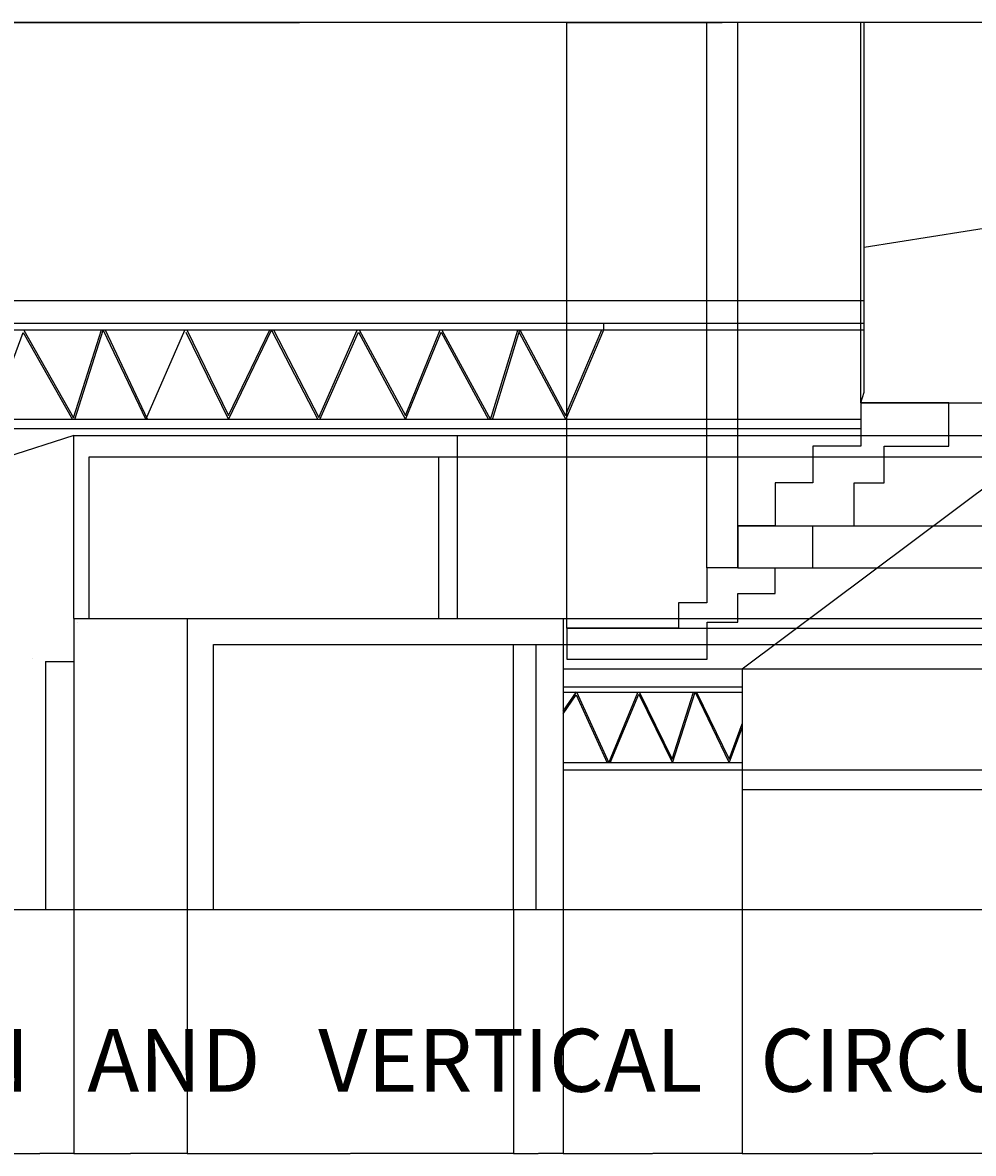
# Model space of a CAD drawing. Units: inches. Extents: x -32109 to 33221, y -19197 to 7608.
# Tile 24 of 25: x 19011 to 26633, y -13530 to -4467. Entities that reach past the tile are written whole.
import ezdxf

# ---------------------------------------------------------------- set-up
doc = ezdxf.new("R2010")
doc.units = ezdxf.units.IN
doc.header["$MEASUREMENT"] = 0
for name, color, linetype, lineweight in [('A-ANNO-DIMS', 2, 'Continuous', 18), ('A-ANNO-TEXT', 7, 'Continuous', 25), ('A-ELEV', 7, 'Continuous', 25)]:
    doc.layers.add(name, color=color, linetype=linetype, lineweight=lineweight)
doc.styles.get("Standard").update_dxf_attribs({"font": 'arial.ttf'})
doc.dimstyles.get("Standard").update_dxf_attribs({"dimtxt": 0.18, "dimasz": 0.18, "dimexe": 0.18, "dimexo": 0.0625, "dimgap": 0.09, "dimtad": 0, "dimtih": 1, "dimtoh": 1, "dimdec": 4, "dimzin": 0, "dimdsep": 46, "dimtxsty": 'Standard', "dimcen": 0.09, "dimadec": 0, "dimazin": 0, "dimtfac": 1, "dimtdec": 4, "dimtofl": 0, "dimtmove": 0, "dimatfit": 3, "dimfxl": 1, "dimtolj": 1, "dimtzin": 0, "dimarcsym": 0})

# ---------------------------------------------------------------- blocks, each defined once
blk = doc.blocks.new('*D16')
at = {"layer": 'A-ANNO-DIMS', "color": 0, "lineweight": -2, "transparency": 16777216}
for p, q in [((7931.85712, -8929.002357), (7931.85712, -4467.086268999999)), ((7932.03712, -4467.266268999999), (18774.66361096794, -4467.266268999999)), ((29618.150443, -4467.266268999999), (18775.52395203206, -4467.266268999999)), ((29618.330443, -6090.731526999999), (29618.330443, -4467.086268999999))]:
    blk.add_line(p, q, dxfattribs=at)
at = {"layer": 'A-ANNO-DIMS', "color": 0, "transparency": 16777216}
for points in [[(7932.03712, -4467.236268999999), (7932.03712, -4467.296269), (7931.85712, -4467.266268999999)], [(29618.150443, -4467.236268999999), (29618.150443, -4467.296269), (29618.330443, -4467.266268999999)]]:
    blk.add_solid(points, dxfattribs=at)
at = {"layer": 'Defpoints', "color": 0, "transparency": 16777216}
for p in [(29618.330443, -4467.266268999999), (29618.330443, -6090.794027), (7931.85712, -8929.064857)]:
    blk.add_point(p, dxfattribs=at)
at = {"layer": 'A-ANNO-DIMS', "color": 0, "transparency": 16777216, "insert": (18775.0937815, -4467.266268999999), "char_height": 0.18, "attachment_point": 5}
blk.add_mtext('\\A1;21686', dxfattribs=at)
blk = doc.blocks.new('*D17')
at = {"layer": 'A-ANNO-DIMS', "color": 0, "lineweight": -2, "transparency": 16777216}
for p, q in [((29618.39294300002, -6090.794027000002), (33221.11530000003, -6090.794027000001)), ((33220.93530000003, -6090.974027000001), (33220.93530000003, -8833.116883862214)), ((33220.93530000003, -11575.623547), (33220.93530000003, -8833.48069013779)), ((8978.174905000003, -11575.803547), (33221.11530000003, -11575.803547))]:
    blk.add_line(p, q, dxfattribs=at)
at = {"layer": 'A-ANNO-DIMS', "color": 0, "transparency": 16777216}
for points in [[(33220.90530000003, -6090.974027000001), (33220.96530000003, -6090.974027000001), (33220.93530000003, -6090.794027000001)], [(33220.90530000003, -11575.623547), (33220.96530000003, -11575.623547), (33220.93530000003, -11575.803547)]]:
    blk.add_solid(points, dxfattribs=at)
at = {"layer": 'Defpoints', "color": 0, "transparency": 16777216}
for p in [(29618.33044300001, -6090.794027000002), (8978.112405000002, -11575.803547), (33220.93530000003, -11575.803547)]:
    blk.add_point(p, dxfattribs=at)
at = {"layer": 'A-ANNO-DIMS', "color": 0, "transparency": 16777216, "insert": (33220.93530000002, -8833.298787000009), "char_height": 0.18, "attachment_point": 5}
blk.add_mtext('\\A1;5485', dxfattribs=at)
blk = doc.blocks.new('*D19')
at = {"layer": 'A-ANNO-DIMS', "color": 0, "lineweight": -2, "transparency": 16777216}
for p, q in [((16706.691851, -6693.317283999999), (16706.691851, -4467.086268999999)), ((16706.871851, -4467.266268999999), (21231.63312013711, -4467.266268999999)), ((25757.077186, -4467.266268999999), (21232.31591686289, -4467.266268999999)), ((25757.257186, -6693.317283999999), (25757.257186, -4467.086268999999))]:
    blk.add_line(p, q, dxfattribs=at)
at = {"layer": 'A-ANNO-DIMS', "color": 0, "transparency": 16777216}
for points in [[(16706.871851, -4467.236268999999), (16706.871851, -4467.296269), (16706.691851, -4467.266268999999)], [(25757.077186, -4467.236268999999), (25757.077186, -4467.296269), (25757.257186, -4467.266268999999)]]:
    blk.add_solid(points, dxfattribs=at)
at = {"layer": 'Defpoints', "color": 0, "transparency": 16777216}
for p in [(25757.257186, -4467.266268999999), (16706.691851, -6693.379784), (25757.257186, -6693.379784)]:
    blk.add_point(p, dxfattribs=at)
at = {"layer": 'A-ANNO-DIMS', "color": 0, "transparency": 16777216, "insert": (21231.9745185, -4467.266268999999), "char_height": 0.18, "attachment_point": 5}
blk.add_mtext('\\A1;9051', dxfattribs=at)
blk = doc.blocks.new('*D135')
at = {"layer": 'A-ANNO-DIMS', "color": 0, "lineweight": -2, "transparency": 16777216}
for p, q in [((18874.369867, -11575.866047), (18874.369867, -13529.670166)), ((19422.73076, -11575.866047), (19422.73076, -13529.670166)), ((18874.549867, -13529.490166), (19148.1569778929, -13529.490166)), ((19422.55076, -13529.490166), (19148.94364910709, -13529.490166))]:
    blk.add_line(p, q, dxfattribs=at)
at = {"layer": 'A-ANNO-DIMS', "color": 0, "transparency": 16777216}
for points in [[(18874.549867, -13529.460166), (18874.549867, -13529.520166), (18874.369867, -13529.490166)], [(19422.55076, -13529.460166), (19422.55076, -13529.520166), (19422.73076, -13529.490166)]]:
    blk.add_solid(points, dxfattribs=at)
at = {"layer": 'Defpoints', "color": 0, "transparency": 16777216}
for p in [(18874.369867, -11575.803547), (19422.73076, -11575.803547), (19422.73076, -13529.490166)]:
    blk.add_point(p, dxfattribs=at)
at = {"layer": 'A-ANNO-DIMS', "color": 0, "transparency": 16777216, "insert": (19148.5503135, -13529.490166), "char_height": 0.18, "attachment_point": 5}
blk.add_mtext('\\A1;548.4', dxfattribs=at)
blk = doc.blocks.new('*D136')
at = {"layer": 'A-ANNO-DIMS', "color": 0, "lineweight": -2, "transparency": 16777216}
for p, q in [((19422.73076, -11575.866047), (19422.73076, -13529.670166)), ((20329.957332, -11575.866047), (20329.957332, -13529.670166)), ((19422.91076, -13529.490166), (19875.95126291678, -13529.490166)), ((20329.777332, -13529.490166), (19876.73682908321, -13529.490166))]:
    blk.add_line(p, q, dxfattribs=at)
at = {"layer": 'A-ANNO-DIMS', "color": 0, "transparency": 16777216}
for points in [[(19422.91076, -13529.460166), (19422.91076, -13529.520166), (19422.73076, -13529.490166)], [(20329.777332, -13529.460166), (20329.777332, -13529.520166), (20329.957332, -13529.490166)]]:
    blk.add_solid(points, dxfattribs=at)
at = {"layer": 'Defpoints', "color": 0, "transparency": 16777216}
for p in [(19422.73076, -11575.803547), (20329.957332, -11575.803547), (20329.957332, -13529.490166)]:
    blk.add_point(p, dxfattribs=at)
at = {"layer": 'A-ANNO-DIMS', "color": 0, "transparency": 16777216, "insert": (19876.34404599999, -13529.490166), "char_height": 0.18, "attachment_point": 5}
blk.add_mtext('\\A1;907.2', dxfattribs=at)
blk = doc.blocks.new('*D137')
at = {"layer": 'A-ANNO-DIMS', "color": 0, "lineweight": -2, "transparency": 16777216}
for p, q in [((20329.957332, -11575.866047), (20329.957332, -13529.670166)), ((22946.308176, -11575.866047), (22946.308176, -13529.670166)), ((20330.137332, -13529.490166), (21637.66795863847, -13529.490166)), ((22946.128176, -13529.490166), (21638.59754936153, -13529.490166))]:
    blk.add_line(p, q, dxfattribs=at)
at = {"layer": 'A-ANNO-DIMS', "color": 0, "transparency": 16777216}
for points in [[(20330.137332, -13529.460166), (20330.137332, -13529.520166), (20329.957332, -13529.490166)], [(22946.128176, -13529.460166), (22946.128176, -13529.520166), (22946.308176, -13529.490166)]]:
    blk.add_solid(points, dxfattribs=at)
at = {"layer": 'Defpoints', "color": 0, "transparency": 16777216}
for p in [(20329.957332, -11575.803547), (22946.308176, -11575.803547), (22946.308176, -13529.490166)]:
    blk.add_point(p, dxfattribs=at)
at = {"layer": 'A-ANNO-DIMS', "color": 0, "transparency": 16777216, "insert": (21638.132754, -13529.490166), "char_height": 0.18, "attachment_point": 5}
blk.add_mtext('\\A1;2616.4', dxfattribs=at)
blk = doc.blocks.new('*D138')
at = {"layer": 'A-ANNO-DIMS', "color": 0, "lineweight": -2, "transparency": 16777216}
for p, q in [((22946.308176, -11575.866047), (22946.308176, -13529.670166)), ((23344.222367, -11575.866047), (23344.222367, -13529.670166)), ((22946.488176, -13529.490166), (23144.87144476057, -13529.490166)), ((23344.042367, -13529.490166), (23145.65909823943, -13529.490166))]:
    blk.add_line(p, q, dxfattribs=at)
at = {"layer": 'A-ANNO-DIMS', "color": 0, "transparency": 16777216}
for points in [[(22946.488176, -13529.460166), (22946.488176, -13529.520166), (22946.308176, -13529.490166)], [(23344.042367, -13529.460166), (23344.042367, -13529.520166), (23344.222367, -13529.490166)]]:
    blk.add_solid(points, dxfattribs=at)
at = {"layer": 'Defpoints', "color": 0, "transparency": 16777216}
for p in [(22946.308176, -11575.803547), (23344.222367, -11575.803547), (23344.222367, -13529.490166)]:
    blk.add_point(p, dxfattribs=at)
at = {"layer": 'A-ANNO-DIMS', "color": 0, "transparency": 16777216, "insert": (23145.2652715, -13529.490166), "char_height": 0.18, "attachment_point": 5}
blk.add_mtext('\\A1;397.9', dxfattribs=at)
blk = doc.blocks.new('*D139')
at = {"layer": 'A-ANNO-DIMS', "color": 0, "lineweight": -2, "transparency": 16777216}
for p, q in [((23344.222367, -11575.866047), (23344.222367, -13529.670166)), ((24779.369992, -11575.866047), (24779.369992, -13529.670166)), ((23344.402367, -13529.490166), (24061.35839641678, -13529.490166)), ((24779.189992, -13529.490166), (24062.23396258322, -13529.490166))]:
    blk.add_line(p, q, dxfattribs=at)
at = {"layer": 'A-ANNO-DIMS', "color": 0, "transparency": 16777216}
for points in [[(23344.402367, -13529.460166), (23344.402367, -13529.520166), (23344.222367, -13529.490166)], [(24779.189992, -13529.460166), (24779.189992, -13529.520166), (24779.369992, -13529.490166)]]:
    blk.add_solid(points, dxfattribs=at)
at = {"layer": 'Defpoints', "color": 0, "transparency": 16777216}
for p in [(23344.222367, -11575.803547), (24779.369992, -11575.803547), (24779.369992, -13529.490166)]:
    blk.add_point(p, dxfattribs=at)
at = {"layer": 'A-ANNO-DIMS', "color": 0, "transparency": 16777216, "insert": (24061.7961795, -13529.490166), "char_height": 0.18, "attachment_point": 5}
blk.add_mtext('\\A1;1435.1', dxfattribs=at)
blk = doc.blocks.new('*D140')
at = {"layer": 'A-ANNO-DIMS', "color": 0, "lineweight": -2, "transparency": 16777216}
for p, q in [((24779.369992, -11575.866047), (24779.369992, -13529.670166)), ((26872.591633, -11575.866047), (26872.591633, -13529.670166)), ((24779.549992, -13529.490166), (25825.51656966234, -13529.490166)), ((26872.411633, -13529.490166), (25826.44505533765, -13529.490166))]:
    blk.add_line(p, q, dxfattribs=at)
at = {"layer": 'A-ANNO-DIMS', "color": 0, "transparency": 16777216}
for points in [[(24779.549992, -13529.460166), (24779.549992, -13529.520166), (24779.369992, -13529.490166)], [(26872.411633, -13529.460166), (26872.411633, -13529.520166), (26872.591633, -13529.490166)]]:
    blk.add_solid(points, dxfattribs=at)
at = {"layer": 'Defpoints', "color": 0, "transparency": 16777216}
for p in [(24779.369992, -11575.803547), (26872.591633, -11575.803547), (26872.591633, -13529.490166)]:
    blk.add_point(p, dxfattribs=at)
at = {"layer": 'A-ANNO-DIMS', "color": 0, "transparency": 16777216, "insert": (25825.9808125, -13529.490166), "char_height": 0.18, "attachment_point": 5}
blk.add_mtext('\\A1;2093.2', dxfattribs=at)
blk = doc.blocks.new('*D142')
at = {"layer": 'A-ANNO-DIMS', "color": 0, "lineweight": -2, "transparency": 16777216}
for p, q in [((19422.79326, -7777.039673000004), (33221.11530000003, -7777.039673000001)), ((33220.93530000003, -7777.219673000002), (33220.93530000003, -9676.23964547067)), ((33220.93530000003, -11575.623547), (33220.93530000003, -9676.603574529332)), ((19422.79326, -11575.803547), (33221.11530000003, -11575.803547))]:
    blk.add_line(p, q, dxfattribs=at)
at = {"layer": 'A-ANNO-DIMS', "color": 0, "transparency": 16777216}
for points in [[(33220.90530000003, -7777.219673000002), (33220.96530000003, -7777.219673000002), (33220.93530000003, -7777.039673000001)], [(33220.90530000003, -11575.623547), (33220.96530000003, -11575.623547), (33220.93530000003, -11575.803547)]]:
    blk.add_solid(points, dxfattribs=at)
at = {"layer": 'Defpoints', "color": 0, "transparency": 16777216}
for p in [(19422.73076, -7777.039673000004), (19422.73076, -11575.803547), (33220.93530000003, -11575.803547)]:
    blk.add_point(p, dxfattribs=at)
at = {"layer": 'A-ANNO-DIMS', "color": 0, "transparency": 16777216, "insert": (33220.93530000002, -9676.421610000009), "char_height": 0.18, "attachment_point": 5}
blk.add_mtext('\\A1;3799', dxfattribs=at)
blk = doc.blocks.new('*D143')
at = {"layer": 'A-ANNO-DIMS', "color": 0, "lineweight": -2, "transparency": 16777216}
for p, q in [((23344.28486700001, -9241.758819000004), (33221.11530000003, -9241.758819000002)), ((33220.93530000003, -9241.938819000003), (33220.93530000003, -10408.59921847067)), ((33220.93530000003, -11575.623547), (33220.93530000003, -10408.96314752933)), ((23344.28486700001, -11575.803547), (33221.11530000003, -11575.803547))]:
    blk.add_line(p, q, dxfattribs=at)
at = {"layer": 'A-ANNO-DIMS', "color": 0, "transparency": 16777216}
for points in [[(33220.90530000003, -9241.938819000003), (33220.96530000003, -9241.938819000003), (33220.93530000003, -9241.758819000002)], [(33220.90530000003, -11575.623547), (33220.96530000003, -11575.623547), (33220.93530000003, -11575.803547)]]:
    blk.add_solid(points, dxfattribs=at)
at = {"layer": 'Defpoints', "color": 0, "transparency": 16777216}
for p in [(23344.222367, -9241.758819000004), (23344.222367, -11575.803547), (33220.93530000003, -11575.803547)]:
    blk.add_point(p, dxfattribs=at)
at = {"layer": 'A-ANNO-DIMS', "color": 0, "transparency": 16777216, "insert": (33220.93530000002, -10408.78118300001), "char_height": 0.18, "attachment_point": 5}
blk.add_mtext('\\A1;2334', dxfattribs=at)
blk = doc.blocks.new('*D144')
at = {"layer": 'A-ANNO-DIMS', "color": 0, "lineweight": -2, "transparency": 16777216}
for p, q in [((22344.03431300001, -7946.222949000004), (33221.11530000003, -7946.222949000001)), ((33220.93530000003, -7946.402949000002), (33220.93530000003, -8593.808980862214)), ((33220.93530000003, -9241.578819000002), (33220.93530000003, -8594.172787137792)), ((22344.03431300001, -9241.758819000004), (33221.11530000003, -9241.758819000002))]:
    blk.add_line(p, q, dxfattribs=at)
at = {"layer": 'A-ANNO-DIMS', "color": 0, "transparency": 16777216}
for points in [[(33220.90530000003, -7946.402949000002), (33220.96530000003, -7946.402949000002), (33220.93530000003, -7946.222949000001)], [(33220.90530000003, -9241.578819000002), (33220.96530000003, -9241.578819000002), (33220.93530000003, -9241.758819000002)]]:
    blk.add_solid(points, dxfattribs=at)
at = {"layer": 'Defpoints', "color": 0, "transparency": 16777216}
for p in [(22343.97181300001, -7946.222949000004), (22343.97181300001, -9241.758819000004), (33220.93530000003, -9241.758819000002)]:
    blk.add_point(p, dxfattribs=at)
at = {"layer": 'A-ANNO-DIMS', "color": 0, "transparency": 16777216, "insert": (33220.93530000002, -8593.99088400001), "char_height": 0.18, "attachment_point": 5}
blk.add_mtext('\\A1;1295.5', dxfattribs=at)
blk = doc.blocks.new('*D145')
at = {"layer": 'A-ANNO-DIMS', "color": 0, "lineweight": -2, "transparency": 16777216}
for p, q in [((20542.28536700001, -9450.896666000002), (33221.11530000003, -9450.896666000002)), ((33220.93530000003, -9451.076666000004), (33220.93530000003, -10513.16820336221)), ((33220.93530000003, -11575.623547), (33220.93530000003, -10513.53200963779)), ((20542.28536700001, -11575.803547), (33221.11530000003, -11575.803547))]:
    blk.add_line(p, q, dxfattribs=at)
at = {"layer": 'A-ANNO-DIMS', "color": 0, "transparency": 16777216}
for points in [[(33220.90530000003, -9451.076666000004), (33220.96530000003, -9451.076666000004), (33220.93530000003, -9450.896666000002)], [(33220.90530000003, -11575.623547), (33220.96530000003, -11575.623547), (33220.93530000003, -11575.803547)]]:
    blk.add_solid(points, dxfattribs=at)
at = {"layer": 'Defpoints', "color": 0, "transparency": 16777216}
for p in [(20542.22286700001, -9450.896666000002), (20542.22286700001, -11575.803547), (33220.93530000003, -11575.803547)]:
    blk.add_point(p, dxfattribs=at)
at = {"layer": 'A-ANNO-DIMS', "color": 0, "transparency": 16777216, "insert": (33220.93530000002, -10513.35010650001), "char_height": 0.18, "attachment_point": 5}
blk.add_mtext('\\A1;2125', dxfattribs=at)
blk = doc.blocks.new('*D146')
at = {"layer": 'A-ANNO-DIMS', "color": 0, "lineweight": -2, "transparency": 16777216}
for p, q in [((23373.7718, -9319.792458), (23373.7718, -4467.086268999999)), ((23373.9518, -4467.266268999999), (24550.92569716235, -4467.266268999999)), ((25728.82808, -4467.266268999999), (24551.85418283766, -4467.266268999999)), ((25729.00808, -7514.295351), (25729.00808, -4467.086268999999))]:
    blk.add_line(p, q, dxfattribs=at)
at = {"layer": 'A-ANNO-DIMS', "color": 0, "transparency": 16777216}
for points in [[(23373.9518, -4467.236268999999), (23373.9518, -4467.296269), (23373.7718, -4467.266268999999)], [(25728.82808, -4467.236268999999), (25728.82808, -4467.296269), (25729.00808, -4467.266268999999)]]:
    blk.add_solid(points, dxfattribs=at)
at = {"layer": 'Defpoints', "color": 0, "transparency": 16777216}
for p in [(25729.00808, -4467.266268999999), (25729.00808, -7514.357850999999), (23373.7718, -9319.854958)]:
    blk.add_point(p, dxfattribs=at)
at = {"layer": 'A-ANNO-DIMS', "color": 0, "transparency": 16777216, "insert": (24551.38994, -4467.266268999999), "char_height": 0.18, "attachment_point": 5}
blk.add_mtext('\\A1;2355.2', dxfattribs=at)
blk = doc.blocks.new('*D147')
at = {"layer": 'A-ANNO-DIMS', "color": 0, "lineweight": -2, "transparency": 16777216}
for p, q in [((25729.07058000001, -7514.357851000004), (33221.11530000003, -7514.357851000003)), ((33220.93530000003, -7514.537851000003), (33220.93530000003, -8416.924501362213)), ((33220.93530000003, -9319.674958000001), (33220.93530000003, -8417.288307637791)), ((23373.8343, -9319.854958000004), (33221.11530000003, -9319.854958000002))]:
    blk.add_line(p, q, dxfattribs=at)
at = {"layer": 'A-ANNO-DIMS', "color": 0, "transparency": 16777216}
for points in [[(33220.90530000003, -7514.537851000003), (33220.96530000003, -7514.537851000003), (33220.93530000003, -7514.357851000003)], [(33220.90530000003, -9319.674958000001), (33220.96530000003, -9319.674958000001), (33220.93530000003, -9319.854958000002)]]:
    blk.add_solid(points, dxfattribs=at)
at = {"layer": 'Defpoints', "color": 0, "transparency": 16777216}
for p in [(25729.00808000002, -7514.357851000004), (33220.93530000003, -7514.357851000003), (23373.77180000001, -9319.854958000004)]:
    blk.add_point(p, dxfattribs=at)
at = {"layer": 'A-ANNO-DIMS', "color": 0, "transparency": 16777216, "insert": (33220.93530000002, -8417.10640450001), "char_height": 0.18, "attachment_point": 5}
blk.add_mtext('\\A1;1805.5', dxfattribs=at)
blk = doc.blocks.new('*D148')
at = {"layer": 'A-ANNO-DIMS', "color": 0, "lineweight": -2, "transparency": 16777216}
for p, q in [((24496.74828, -8835.455653000003), (24496.74828, -4467.086268999999)), ((24496.92828, -4467.266268999999), (24619.50049278922, -4467.266268999999)), ((24743.003033, -4467.266268999999), (24620.43082021078, -4467.266268999999)), ((24743.183033, -8835.455653000003), (24743.183033, -4467.086268999999))]:
    blk.add_line(p, q, dxfattribs=at)
at = {"layer": 'A-ANNO-DIMS', "color": 0, "transparency": 16777216}
for points in [[(24496.92828, -4467.236268999999), (24496.92828, -4467.296269), (24496.74828, -4467.266268999999)], [(24743.003033, -4467.236268999999), (24743.003033, -4467.296269), (24743.183033, -4467.266268999999)]]:
    blk.add_solid(points, dxfattribs=at)
at = {"layer": 'Defpoints', "color": 0, "transparency": 16777216}
for p in [(24743.183033, -4467.266268999999), (24496.74828, -8835.518153), (24743.183033, -8835.518153)]:
    blk.add_point(p, dxfattribs=at)
at = {"layer": 'A-ANNO-DIMS', "color": 0, "transparency": 16777216, "insert": (24619.9656565, -4467.266268999999), "char_height": 0.18, "attachment_point": 5}
blk.add_mtext('\\A1;246.43', dxfattribs=at)
blk = doc.blocks.new('*D149')
at = {"layer": 'A-ANNO-DIMS', "color": 0, "lineweight": -2, "transparency": 16777216}
for p, q in [((24743.24553300002, -8499.326661000003), (33221.11530000003, -8499.326661000001)), ((33220.93530000003, -8499.506661000001), (33220.93530000003, -8667.240442470671)), ((33220.93530000003, -8835.338153000002), (33220.93530000003, -8667.604371529334)), ((24743.24553300002, -8835.518153000005), (33221.11530000003, -8835.518153000003))]:
    blk.add_line(p, q, dxfattribs=at)
at = {"layer": 'A-ANNO-DIMS', "color": 0, "transparency": 16777216}
for points in [[(33220.90530000003, -8499.506661000001), (33220.96530000003, -8499.506661000001), (33220.93530000003, -8499.326661000001)], [(33220.90530000003, -8835.338153000002), (33220.96530000003, -8835.338153000002), (33220.93530000003, -8835.518153000003)]]:
    blk.add_solid(points, dxfattribs=at)
at = {"layer": 'Defpoints', "color": 0, "transparency": 16777216}
for p in [(24743.18303300002, -8499.326661000003), (33220.93530000003, -8499.326661000001), (24743.18303300002, -8835.518153000005)]:
    blk.add_point(p, dxfattribs=at)
at = {"layer": 'A-ANNO-DIMS', "color": 0, "transparency": 16777216, "insert": (33220.93530000002, -8667.422407000007), "char_height": 0.18, "attachment_point": 5}
blk.add_mtext('\\A1;336.2', dxfattribs=at)
blk = doc.blocks.new('*D150')
at = {"layer": 'A-ANNO-DIMS', "color": 0, "lineweight": -2, "transparency": 16777216}
for p, q in [((24779.43249200002, -9646.283758000003), (33221.11530000003, -9646.283758000001)), ((33220.93530000003, -9646.463758000002), (33220.93530000003, -10050.72724947067)), ((33220.93530000003, -10455.35467), (33220.93530000003, -10051.09117852933)), ((24779.43249200002, -10455.53467), (33221.11530000003, -10455.53467))]:
    blk.add_line(p, q, dxfattribs=at)
at = {"layer": 'A-ANNO-DIMS', "color": 0, "transparency": 16777216}
for points in [[(33220.90530000003, -9646.463758000002), (33220.96530000003, -9646.463758000002), (33220.93530000003, -9646.283758000001)], [(33220.90530000003, -10455.35467), (33220.96530000003, -10455.35467), (33220.93530000003, -10455.53467)]]:
    blk.add_solid(points, dxfattribs=at)
at = {"layer": 'Defpoints', "color": 0, "transparency": 16777216}
for p in [(24779.36999200001, -9646.283758000003), (24779.36999200001, -10455.53467), (33220.93530000003, -10455.53467)]:
    blk.add_point(p, dxfattribs=at)
at = {"layer": 'A-ANNO-DIMS', "color": 0, "transparency": 16777216, "insert": (33220.93530000002, -10050.90921400001), "char_height": 0.18, "attachment_point": 5}
blk.add_mtext('\\A1;809.3', dxfattribs=at)
blk = doc.blocks.new('*D151')
at = {"layer": 'A-ANNO-DIMS', "color": 0, "lineweight": -2, "transparency": 16777216}
for p, q in [((24779.43249200002, -10455.53467), (33221.11530000003, -10455.53467)), ((33220.93530000003, -10455.71467), (33220.93530000003, -11015.48714397067)), ((33220.93530000003, -11575.623547), (33220.93530000003, -11015.85107302933)), ((24779.43249200002, -11575.803547), (33221.11530000003, -11575.803547))]:
    blk.add_line(p, q, dxfattribs=at)
at = {"layer": 'A-ANNO-DIMS', "color": 0, "transparency": 16777216}
for points in [[(33220.90530000003, -10455.71467), (33220.96530000003, -10455.71467), (33220.93530000003, -10455.53467)], [(33220.90530000003, -11575.623547), (33220.96530000003, -11575.623547), (33220.93530000003, -11575.803547)]]:
    blk.add_solid(points, dxfattribs=at)
at = {"layer": 'Defpoints', "color": 0, "transparency": 16777216}
for p in [(24779.36999200001, -10455.53467), (24779.36999200001, -11575.803547), (33220.93530000003, -11575.803547)]:
    blk.add_point(p, dxfattribs=at)
at = {"layer": 'A-ANNO-DIMS', "color": 0, "transparency": 16777216, "insert": (33220.93530000002, -11015.66910850001), "char_height": 0.18, "attachment_point": 5}
blk.add_mtext('\\A1;1120.3', dxfattribs=at)

msp = doc.modelspace()

# ---------------------------------------------------------------- linework, layer by layer
at = {"layer": 'A-ELEV'}
for p, q in [((25757.25718631681, -6267.046394138653), (26872.59163338689, -6090.794027193029)), ((25757.25718631681, -7429.041241976618), (25757.25718631681, -6267.046394138653)), ((16706.69185113072, -6693.379783521264), (25757.25718631681, -6693.379783521264)), ((25757.25718631681, -6878.434109803435), (16706.69185113072, -6878.434109803435)), ((23669.24763625898, -6930.59382918874), (23669.24763625898, -6878.434109803435)), ((16706.69185113072, -6930.59382918874), (25757.25718631681, -6930.593829188739)), ((18756.5328218629, -7648.26031267421), (19015.149545349, -6949.672977624011)), ((19015.149545349, -6949.672977624015), (19411.55462750871, -7648.022736218671)), ((19021.66471751541, -6932.073896250702), (19419.77536563133, -7633.428362976982)), ((19419.77536563133, -7633.428362976982), (19642.36133175424, -6930.59382918874)), ((19430.209726088, -7648.022736218671), (19657.11379919641, -6931.553404321356)), ((19657.11379919641, -6931.553404321356), (19997.80615847221, -7648.395624455301)), ((19672.55012575191, -6930.59382918874), (20010.77021950304, -7642.23421764312)), ((19997.80615847221, -7648.395624455301), (20311.54213373321, -6931.648918519761)), ((20319.78875044917, -6948.604857041963), (20660.17657549292, -7648.479149002222)), ((20326.99032840441, -6930.59382918874), (20660.14304566561, -7615.591954717591)), ((20660.14304566561, -7615.591954717594), (20991.57031184739, -6930.59382918874)), ((20660.17657549292, -7648.479149002222), (21006.9265580369, -6931.811836725292)), ((21006.9265580369, -6931.811836725292), (21378.03932263788, -7648.554613279255)), ((21022.45959341933, -6930.59382918874), (21385.47255796398, -7631.693184832212)), ((21385.47255796398, -7631.693184832212), (21693.96096490137, -6931.923169203415)), ((21393.96041812104, -7648.022736218671), (21702.60191292903, -6947.905458588476)), ((21702.60191292903, -6947.905458588476), (22081.42406820136, -7648.57456244727)), ((21709.55955507691, -6930.59382918874), (22079.57910689063, -7614.981645928674)), ((22079.57910689063, -7614.981645928671), (22357.6336928922, -6930.59382918874)), ((22081.42406820136, -7648.57456244727), (22365.69328819586, -6948.890397420449)), ((22365.69328819586, -6948.890397420449), (22745.60385831582, -7648.022736218671)), ((22372.68198414496, -6931.688816855828), (22762.17290364754, -7648.451441824422)), ((22762.17290364754, -7648.451441824422), (22981.67959355174, -6931.585443894231)), ((22777.31574538568, -7648.022736218671), (22996.99479987902, -6930.593829188739)), ((22991.22569560263, -6949.434597531868), (23365.11288978613, -7648.523077473223)), ((22997.42688721696, -6930.59382918874), (23363.60669008725, -7615.271148327359)), ((23363.60669008725, -7615.271148327363), (23653.5546436366, -6930.59382918874)), ((23365.11288978613, -7648.523077473223), (23669.24763625898, -6930.345348253618)), ((25729.00808019247, -7514.357851348876), (25757.25718631681, -7429.041241976618)), ((26171.46601150075, -7514.357851348876), (25729.00808019247, -7514.357851348876)), ((25729.00808019247, -7514.357851348876), (25729.00808019247, -7861.472150721394)), ((26434.91882651764, -7514.357851348876), (26171.46601150075, -7514.357851348876)), ((26434.91882651764, -7861.472150721394), (26434.91882651764, -7514.357851348876)), ((25729.00808019247, -7648.022736218671), (16706.69185113072, -7648.022736218671)), ((21378.03932263788, -7648.554613279255), (21378.27379668426, -7648.022736218671)), ((16706.69185113072, -7719.714605413138), (25729.00808019247, -7719.714605413137)), ((19422.7307598554, -7777.03967259821), (18874.36986664877, -7952.782683843499)), ((19422.7307598554, -9241.758818643346), (19422.7307598554, -7777.03967259821)), ((22495.30366565329, -7777.03967259821), (22495.30366565329, -9241.758818643346)), ((25729.00808019247, -7861.472150721394), (25344.32892339581, -7861.472150721394)), ((25344.32892339581, -7861.472150721394), (25344.32892339581, -8155.639385013335)), ((25916.98108429396, -8155.639385013335), (25916.98108429413, -7861.472150721394)), ((25916.98108429413, -7861.472150721394), (26434.91882651764, -7861.472150721394)), ((19543.29390663711, -9241.758818643346), (19543.29390663711, -7946.222948780469)), ((19543.29390663711, -7946.222948780469), (22343.97181331607, -7946.222948780469)), ((22343.97181331607, -7946.222948780469), (22343.97181331607, -9241.758818643346)), ((24779.36999243395, -9646.283757557641), (26872.5916333869, -8080.142133134835)), ((25344.32892339581, -8155.639385013335), (25043.79793383531, -8155.639385013335)), ((25043.79793383531, -8155.639385013335), (25043.79793383531, -8499.32666072917)), ((25677.02555864514, -8499.32666072917), (25677.02555864514, -8155.639385013335)), ((25677.02555864514, -8155.639385013335), (25916.98108429396, -8155.639385013335)), ((25043.79793383531, -8499.32666072917), (24743.18303297109, -8499.32666072917)), ((24743.18303297109, -8499.32666072917), (24743.18303297109, -8835.51815332094)), ((25345.7054936435, -8835.51815332095), (25345.7054936435, -8499.32666072917)), ((25345.7054936435, -8499.32666072917), (25677.02555864514, -8499.32666072917)), ((24743.18303297109, -8835.51815332094), (24496.7482800759, -8835.51815332094)), ((24496.7482800759, -8835.51815332094), (24496.7482800759, -9118.159023154687)), ((25044.84416971027, -9041.322313003568), (25044.84416971027, -8835.51815332095)), ((25044.84416971027, -8835.51815332095), (25345.7054936435, -8835.51815332095)), ((24743.18303297109, -9271.832443456919), (24743.18303297109, -9041.322313003568)), ((24743.18303297109, -9041.322313003568), (25044.84416971027, -9041.322313003568)), ((24496.7482800759, -9118.159023154687), (24268.06767200416, -9118.159023154687)), ((24268.06767200416, -9118.159023154687), (24268.06767200416, -9319.854958333506)), ((19422.7307598554, -9241.758818643346), (20329.95733241268, -9241.758818643346)), ((19422.7307598554, -9241.758818643346), (19422.7307598554, -9484.978943045822)), ((20329.95733241268, -9241.758818643346), (20329.95733241268, -11575.80354668384)), ((20329.95733241268, -9241.758818643346), (23344.2223674549, -9241.758818643346)), ((23344.2223674549, -9241.758818643346), (23344.2223674549, -11575.80354668384)), ((19449.17297864132, -9278.623716741618), (19449.21427147988, -9278.623716741618)), ((19449.21427147988, -9278.623716741618), (19449.21427147988, -9278.526208655583)), ((24268.06767200416, -9319.854958333506), (23373.77180023778, -9319.854958333506)), ((23373.77180023778, -9319.854958333506), (23373.77180023778, -9569.574266324591)), ((24498.85456001512, -9569.574266324591), (24498.85456001512, -9271.832443456919)), ((24498.85456001512, -9271.832443456919), (24743.18303297109, -9271.832443456919)), ((19422.7307598554, -9484.978943045822), (19422.73075985541, -11575.80354668384)), ((20542.22286703834, -11575.80354668384), (20542.22286703834, -9450.896665734723)), ((20542.22286703834, -9450.896665734723), (23124.62520724542, -9450.896665734723)), ((22946.30817563678, -11575.80354668384), (22946.30817563678, -9450.896665734723)), ((23124.62520724542, -9450.896665734723), (23124.62520724542, -11575.80354668384)), ((19093.31444748436, -9560.154851328736), (19093.17151715826, -9560.154851328734)), ((19193.60640244228, -9588.287943091858), (19193.60640244228, -11575.80354668384)), ((19193.60640244228, -9588.287943091858), (19422.7307598554, -9588.287943091855)), ((23373.77180023778, -9569.574266324591), (24498.85456001512, -9569.574266324591)), ((23344.2223674549, -9646.283757557647), (24779.36999243393, -9646.283757557647)), ((24779.36999243395, -9646.283757557641), (24779.36999243395, -10455.53467010261)), ((24779.36999243395, -9646.283757557641), (24779.36999243395, -11575.80354668383)), ((24779.36999243395, -9792.196552505202), (23344.2223674549, -9792.196552505202)), ((23344.2223674549, -9986.15566482978), (23451.10873564512, -9831.147284610823)), ((23344.2223674549, -9833.323774938168), (24779.36999243395, -9833.323774938168)), ((23344.2223674549, -10006.09262840124), (23449.08371355082, -9854.020968739416)), ((23449.08371355082, -9854.020968739413), (23697.10120669922, -10399.00661577749)), ((23451.10873564512, -9831.147284610823), (23709.62106273317, -10399.19394155008)), ((23709.62106273317, -10399.19394155008), (23943.89797603575, -9835.98859924523)), ((23721.95682693909, -10399.00661577749), (23950.53117572504, -9849.510327238673)), ((23950.53117572504, -9849.510327238673), (24220.1831892418, -10399.19394155008)), ((23954.05894035145, -9831.004051014826), (24217.97442777939, -10368.99379976608)), ((24217.97442777939, -10368.99379976608), (24389.59442707852, -9833.323774938168)), ((24220.1831892418, -10399.19394155008), (24401.14206754539, -9834.374880662202)), ((24401.14206754539, -9834.374880662202), (24675.81154494205, -10399.19394155008)), ((24413.21592531775, -9833.323774938168), (24674.39899938511, -10370.40994851941)), ((24674.39899938511, -10370.40994851941), (24779.36999243395, -10086.8574956731)), ((24675.81154494205, -10399.19394155008), (24779.36999243395, -10119.45712143996)), ((24779.36999243395, -10399.00661577749), (23344.22236745491, -10399.00661577749)), ((23344.2223674549, -10455.53467010261), (24779.36999243395, -10455.53467010262)), ((24779.36999243395, -10455.53467010263), (26632.55012788989, -10455.53467010263)), ((24779.36999243395, -10614.3304611299), (27330.3209813765, -10614.3304611299)), ((6605.539725432871, -11575.80354668384), (31840.93529984972, -11575.80354668384)), ((11053.82493697622, -11575.80354668384), (20871.06445360743, -11575.80354668384)), ((20871.06445360743, -11575.80354668384), (28549.41971044784, -11575.80354668384))]:
    msp.add_line(p, q, dxfattribs=at)

# ---------------------------------------------------------------- texts
at = {"layer": 'A-ANNO-TEXT'}
msp.add_text('SIDE  PROFILE   ATRIUM   CIRCULATION   AND   VERTICAL   CIRCULATION   HUB', height=504.218310670369, dxfattribs=at).set_placement((6653.0921668488, -13035.81166412015))

# ---------------------------------------------------------------- dimensions: what is measured, and where the dimension line sits
at = {"layer": 'A-ANNO-DIMS'}
for base, p1, p2, override, picture, middle in [((29618.330443, -4467.266268999999), (7931.85712, -8929.064857), (29618.330443, -6090.794027), {"dimdec": 0, "dimlfac": 1, "dimrnd": 0, "dimzin": 0, "dimdsep": 46, "dimlunit": 2}, '*D16', (18775.0937815, -4467.266268999999)), ((25757.257186, -4467.266268999999), (16706.691851, -6693.379784), (25757.257186, -6693.379784), {"dimdec": 0, "dimlfac": 1, "dimrnd": 0, "dimzin": 0, "dimdsep": 46, "dimlunit": 2}, '*D19', (21231.9745185, -4467.266268999999)), ((25729.00808, -4467.266268999999), (23373.7718, -9319.854958), (25729.00808, -7514.357850999999), {"dimdec": 1, "dimlfac": 1, "dimrnd": 0, "dimzin": 0, "dimdsep": 46, "dimlunit": 2}, '*D146', (24551.38994, -4467.266268999999)), ((24743.183033, -4467.266268999999), (24496.74828, -8835.518153), (24743.183033, -8835.518153), {"dimdec": 2, "dimlfac": 1, "dimrnd": 0, "dimzin": 0, "dimdsep": 46, "dimlunit": 2}, '*D148', (24619.9656565, -4467.266268999999)), ((19422.73076, -13529.490166), (18874.369867, -11575.803547), (19422.73076, -11575.803547), {"dimdec": 1, "dimlfac": 1, "dimrnd": 0, "dimzin": 0, "dimdsep": 46, "dimlunit": 2}, '*D135', (19148.5503135, -13529.490166)), ((20329.957332, -13529.490166), (19422.73076, -11575.803547), (20329.957332, -11575.803547), {"dimdec": 1, "dimlfac": 1, "dimrnd": 0, "dimzin": 0, "dimdsep": 46, "dimlunit": 2}, '*D136', (19876.34404599999, -13529.490166)), ((22946.308176, -13529.490166), (20329.957332, -11575.803547), (22946.308176, -11575.803547), {"dimdec": 1, "dimlfac": 1, "dimrnd": 0, "dimzin": 0, "dimdsep": 46, "dimlunit": 2}, '*D137', (21638.132754, -13529.490166)), ((23344.222367, -13529.490166), (22946.308176, -11575.803547), (23344.222367, -11575.803547), {"dimdec": 1, "dimlfac": 1, "dimrnd": 0, "dimzin": 0, "dimdsep": 46, "dimlunit": 2}, '*D138', (23145.2652715, -13529.490166)), ((24779.369992, -13529.490166), (23344.222367, -11575.803547), (24779.369992, -11575.803547), {"dimdec": 1, "dimlfac": 1, "dimrnd": 0, "dimzin": 0, "dimdsep": 46, "dimlunit": 2}, '*D139', (24061.7961795, -13529.490166)), ((26872.591633, -13529.490166), (24779.369992, -11575.803547), (26872.591633, -11575.803547), {"dimdec": 1, "dimlfac": 1, "dimrnd": 0, "dimzin": 0, "dimdsep": 46, "dimlunit": 2}, '*D140', (25825.9808125, -13529.490166))]:
    dim = msp.add_linear_dim(base=base, p1=p1, p2=p2, dimstyle='Standard', override=override, dxfattribs=at)
    dim.commit()
    dim.dimension.update_dxf_attribs({"geometry": picture, "text_midpoint": middle})
for base, p1, p2, override, picture, middle in [((33220.93530000003, -11575.803547), (29618.330443, -6090.794027), (8978.112405, -11575.803547), {"dimdec": 0, "dimlfac": 1, "dimrnd": 0, "dimzin": 0, "dimdsep": 46, "dimlunit": 2}, '*D17', (33220.93530000002, -8833.298787000009)), ((33220.93530000003, -7514.357851000003), (23373.7718, -9319.854958), (25729.00808, -7514.357850999999), {"dimdec": 1, "dimlfac": 1, "dimrnd": 0, "dimzin": 0, "dimdsep": 46, "dimlunit": 2}, '*D147', (33220.93530000002, -8417.10640450001)), ((33220.93530000003, -11575.803547), (19422.73076, -7777.039673), (19422.73076, -11575.803547), {"dimdec": 0, "dimlfac": 1, "dimrnd": 0, "dimzin": 0, "dimdsep": 46, "dimlunit": 2}, '*D142', (33220.93530000002, -9676.421610000009)), ((33220.93530000003, -9241.758819000002), (22343.971813, -7946.222949), (22343.971813, -9241.758819), {"dimdec": 1, "dimlfac": 1, "dimrnd": 0, "dimzin": 0, "dimdsep": 46, "dimlunit": 2}, '*D144', (33220.93530000002, -8593.99088400001)), ((33220.93530000003, -8499.326661000001), (24743.183033, -8835.518153), (24743.183033, -8499.326661), {"dimdec": 1, "dimlfac": 1, "dimrnd": 0, "dimzin": 0, "dimdsep": 46, "dimlunit": 2}, '*D149', (33220.93530000002, -8667.422407000007)), ((33220.93530000003, -11575.803547), (23344.222367, -9241.758819), (23344.222367, -11575.803547), {"dimdec": 0, "dimlfac": 1, "dimrnd": 0, "dimzin": 0, "dimdsep": 46, "dimlunit": 2}, '*D143', (33220.93530000002, -10408.78118300001)), ((33220.93530000003, -11575.803547), (20542.222867, -9450.896666), (20542.222867, -11575.803547), {"dimdec": 0, "dimlfac": 1, "dimrnd": 0, "dimzin": 0, "dimdsep": 46, "dimlunit": 2}, '*D145', (33220.93530000002, -10513.35010650001)), ((33220.93530000003, -10455.53467), (24779.369992, -9646.283758), (24779.369992, -10455.53467), {"dimdec": 1, "dimlfac": 1, "dimrnd": 0, "dimzin": 0, "dimdsep": 46, "dimlunit": 2}, '*D150', (33220.93530000002, -10050.90921400001)), ((33220.93530000003, -11575.803547), (24779.369992, -10455.53467), (24779.369992, -11575.803547), {"dimdec": 1, "dimlfac": 1, "dimrnd": 0, "dimzin": 0, "dimdsep": 46, "dimlunit": 2}, '*D151', (33220.93530000002, -11015.66910850001))]:
    dim = msp.add_linear_dim(base=base, p1=p1, p2=p2, angle=90, dimstyle='Standard', override=override, dxfattribs=at)
    dim.commit()
    dim.dimension.update_dxf_attribs({"geometry": picture, "text_midpoint": middle})

doc.saveas('drawing.dxf')
